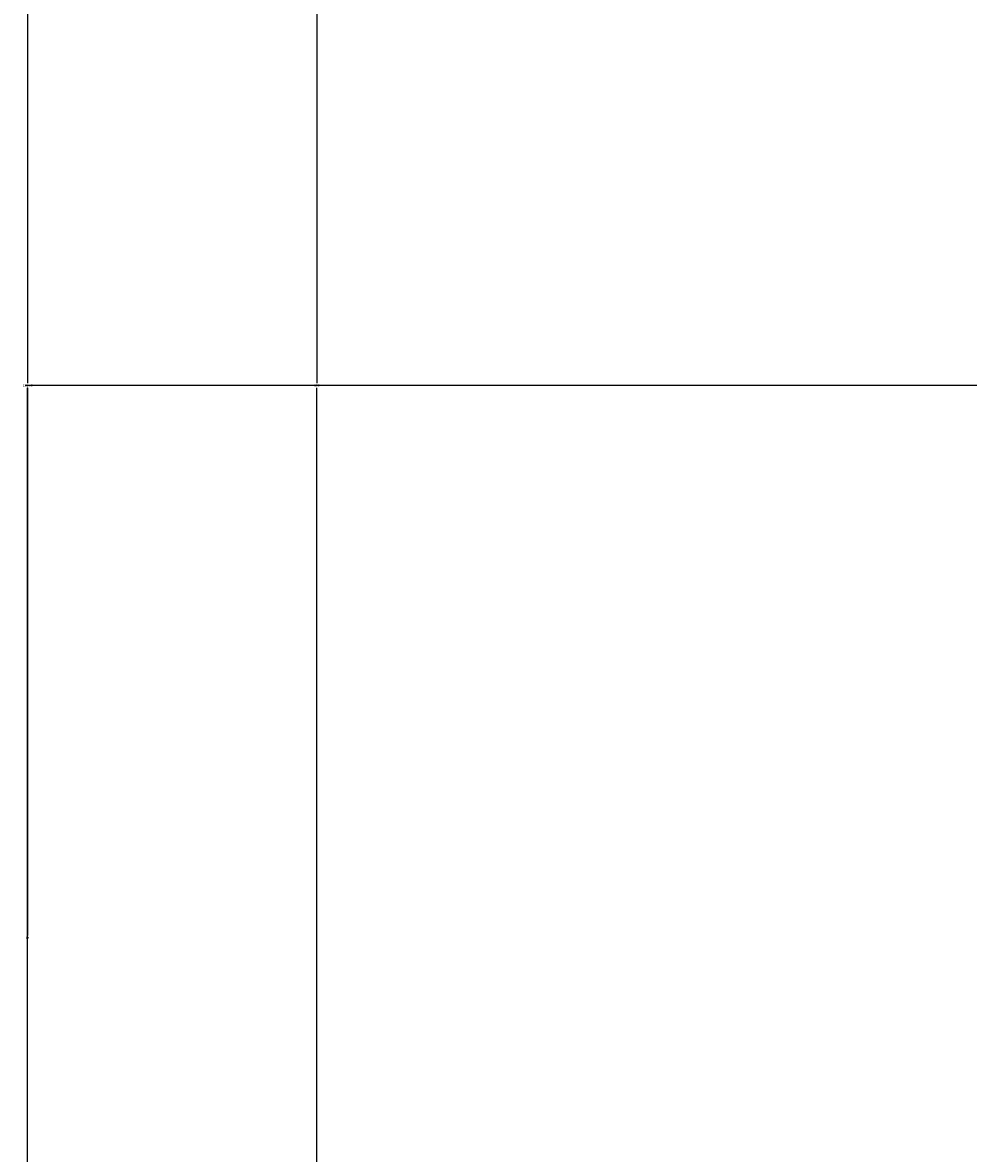
# Model space of a CAD drawing. Units: inches. Extents: x 1095 to 1408, y -20 to 240.
# Tile 3 of 8: x 1095 to 1167, y 66 to 152. Entities that reach past the tile are written whole.
import ezdxf

# ---------------------------------------------------------------- set-up
doc = ezdxf.new("R2010")
doc.units = ezdxf.units.IN
doc.header["$MEASUREMENT"] = 0
doc.layers.add('M-DIMS', color=2, linetype='Continuous', lineweight=18)
doc.styles.get("Standard").update_dxf_attribs({"font": 'arial.ttf'})
doc.dimstyles.get("Standard").update_dxf_attribs({"dimtxt": 0.18, "dimasz": 0.18, "dimexe": 0.18, "dimexo": 0.0625, "dimgap": 0.09, "dimtad": 0, "dimtih": 1, "dimtoh": 1, "dimdec": 4, "dimzin": 0, "dimdsep": 46, "dimtxsty": 'Standard', "dimcen": 0.09, "dimadec": 0, "dimazin": 0, "dimtfac": 1, "dimtdec": 4, "dimtofl": 0, "dimtmove": 0, "dimatfit": 3, "dimfxl": 1, "dimtolj": 1, "dimtzin": 0, "dimarcsym": 0})

# ---------------------------------------------------------------- blocks, each defined once
blk = doc.blocks.new('*D6')
at = {"layer": 'Defpoints', "color": 0, "transparency": 16777216}
for p in [(1117.034, 208), (1137.184, 208), (1137.184, 40)]:
    blk.add_point(p, dxfattribs=at)
at = {"layer": 'M-DIMS', "color": 0, "lineweight": -2, "transparency": 16777216}
for p, q in [((1137.121, 208), (1116.854, 208)), ((1117.034, 207.82), (1117.034, 124.182)), ((1117.034, 40.18), (1117.034, 123.818)), ((1137.121, 40), (1116.854, 40))]:
    blk.add_line(p, q, dxfattribs=at)
at = {"layer": 'M-DIMS', "color": 0, "transparency": 16777216}
for points in [[(1117.004, 207.82), (1117.064, 207.82), (1117.034, 208)], [(1117.004, 40.18), (1117.064, 40.18), (1117.034, 40)]]:
    blk.add_solid(points, dxfattribs=at)
at = {"layer": 'M-DIMS', "color": 0, "transparency": 16777216, "insert": (1117.034, 124), "char_height": 0.18, "attachment_point": 5}
blk.add_mtext('\\A1;168', dxfattribs=at)
blk = doc.blocks.new('*D8')
at = {"layer": 'Defpoints', "color": 0, "transparency": 16777216}
for p in [(1095.034, 124), (1387.184, 124), (1365.184, 40)]:
    blk.add_point(p, dxfattribs=at)
at = {"layer": 'M-DIMS', "color": 0, "lineweight": -2, "transparency": 16777216}
for p, q in [((1387.121, 124), (1094.854, 124)), ((1095.034, 123.82), (1095.034, 82.182)), ((1095.034, 40.18), (1095.034, 81.818)), ((1365.121, 40), (1094.854, 40))]:
    blk.add_line(p, q, dxfattribs=at)
at = {"layer": 'M-DIMS', "color": 0, "transparency": 16777216}
for points in [[(1095.004, 123.82), (1095.064, 123.82), (1095.034, 124)], [(1095.004, 40.18), (1095.064, 40.18), (1095.034, 40)]]:
    blk.add_solid(points, dxfattribs=at)
at = {"layer": 'M-DIMS', "color": 0, "transparency": 16777216, "insert": (1095.034, 82), "char_height": 0.18, "attachment_point": 5}
blk.add_mtext('\\A1;84', dxfattribs=at)
blk = doc.blocks.new('*D10')
at = {"layer": 'Defpoints', "color": 0, "transparency": 16777216}
for p in [(1095.034, 193.282), (1211.184, 193.282), (1211.184, 54.718)]:
    blk.add_point(p, dxfattribs=at)
at = {"layer": 'M-DIMS', "color": 0, "lineweight": -2, "transparency": 16777216}
for p, q in [((1211.121, 193.282), (1094.854, 193.282)), ((1095.034, 193.102), (1095.034, 124.182)), ((1095.034, 54.898), (1095.034, 123.818)), ((1211.121, 54.718), (1094.854, 54.718))]:
    blk.add_line(p, q, dxfattribs=at)
at = {"layer": 'M-DIMS', "color": 0, "transparency": 16777216}
for points in [[(1095.004, 193.102), (1095.064, 193.102), (1095.034, 193.282)], [(1095.004, 54.898), (1095.064, 54.898), (1095.034, 54.718)]]:
    blk.add_solid(points, dxfattribs=at)
at = {"layer": 'M-DIMS', "color": 0, "transparency": 16777216, "insert": (1095.034, 124), "char_height": 0.18, "attachment_point": 5}
blk.add_mtext('\\A1;138.56', dxfattribs=at)

msp = doc.modelspace()

# ---------------------------------------------------------------- dimensions: what is measured, and where the dimension line sits
at = {"layer": 'M-DIMS'}
for base, p1, p2, override, picture, middle in [((1117.034, 208), (1137.184, 40), (1137.184, 208), {"dimdec": 0, "dimlfac": 1, "dimrnd": 0, "dimzin": 0, "dimdsep": 46, "dimlunit": 2}, '*D6', (1117.034, 124)), ((1095.034, 193.282), (1211.184, 54.718), (1211.184, 193.282), {"dimdec": 2, "dimlfac": 1, "dimrnd": 0, "dimzin": 0, "dimdsep": 46, "dimlunit": 2}, '*D10', (1095.034, 124)), ((1095.034, 124), (1365.184, 40), (1387.184, 124), {"dimdec": 0, "dimlfac": 1, "dimrnd": 0, "dimzin": 0, "dimdsep": 46, "dimlunit": 2}, '*D8', (1095.034, 82))]:
    dim = msp.add_linear_dim(base=base, p1=p1, p2=p2, angle=90, dimstyle='Standard', override=override, dxfattribs=at)
    dim.commit()
    dim.dimension.update_dxf_attribs({"geometry": picture, "text_midpoint": middle})

doc.saveas('drawing.dxf')
